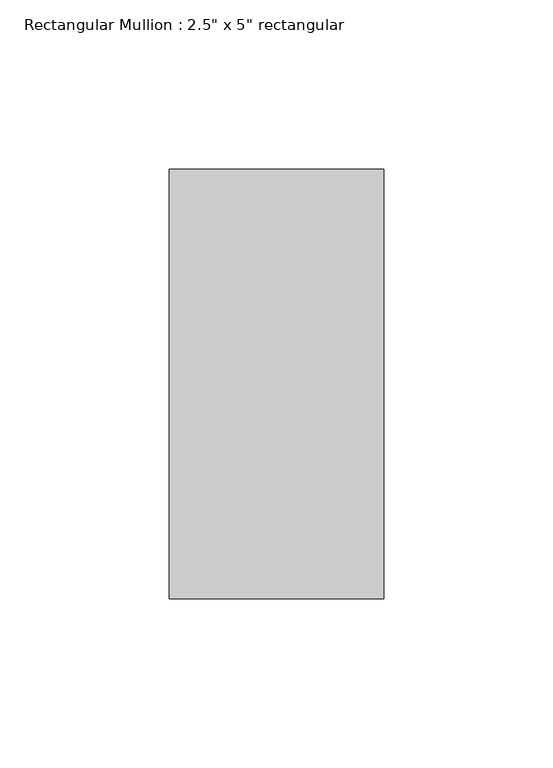
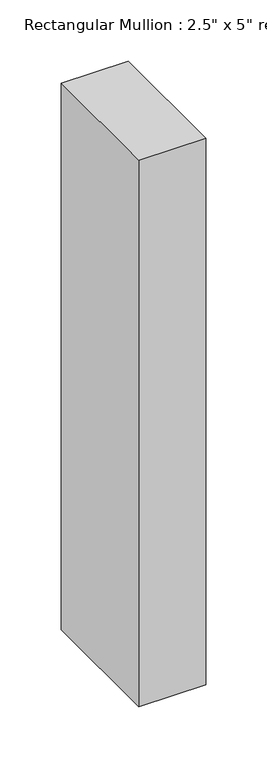
"""IFC4 building model written with IfcOpenShell, lengths in millimetres: member geometry."""

from ifc_helpers import new_model, si_unit, frame, origin, place, context, project, spatial, polyline, outline, extrude, source, transform, mapped, element, save


def member_a980948f(model_context):
    return source(origin(), model_context, "Body", "SweptSolid", [
        extrude(outline(polyline([(0.0, 63.5), (0.0, -63.5), (-63.5, -63.5), (-63.5, 63.5), (0.0, 63.5)])), frame((0.0, 0.0, -546.1), z_axis=(0.0, 0.0, 1.0), x_axis=(1.0, 0.0, 0.0)), (0.0, 0.0, 1.0), 546.1),
    ])


if __name__ == "__main__":
    model = new_model("IFC4")
    model_context = context("Model", 3, world=origin())
    ifc_project = project(units=[si_unit("LENGTHUNIT", "METRE", prefix="MILLI")], contexts=[model_context])
    site = spatial("IfcSite", under=ifc_project)
    building = spatial("IfcBuilding", under=site)
    placement = place(None, origin())
    member_shape = member_a980948f(model_context)
    element("IfcMember", 1, ObjectType="Rectangular Mullion : 2.5\" x 5\" rectangular", at=placement, inside=building, context=model_context, shape_type="MappedRepresentation", body=[
        mapped(member_shape, transform((0.0, 0.0, 0.0), x_axis=(1.0, 0.0, 0.0), y_axis=(0.0, 1.0, 0.0), z_axis=(0.0, 0.0, 1.0))),
    ])
    save(model, "model.ifc")

# Revit data of these elements
# Type "Rectangular Mullion : 2.5\" x 5\" rectangular"
#   built-in parameter 1007304 = 0.416667 (stored number, unit not read)
#   built-in parameter 1007301 = 0.104167 (stored number, unit not read)
#   built-in parameter 1007300 = 0.104167 (stored number, unit not read)
# Element 1 (IfcMember, "Rectangular Mullion : 2.5\" x 5\" rectangular")
#   Materials on its faces: "Aluminum"
# Materials
#   "Aluminum": class "Metal", colour RGB 247 247 247, transparency 0, Description = "Aluminum 6061", Cost = 0
